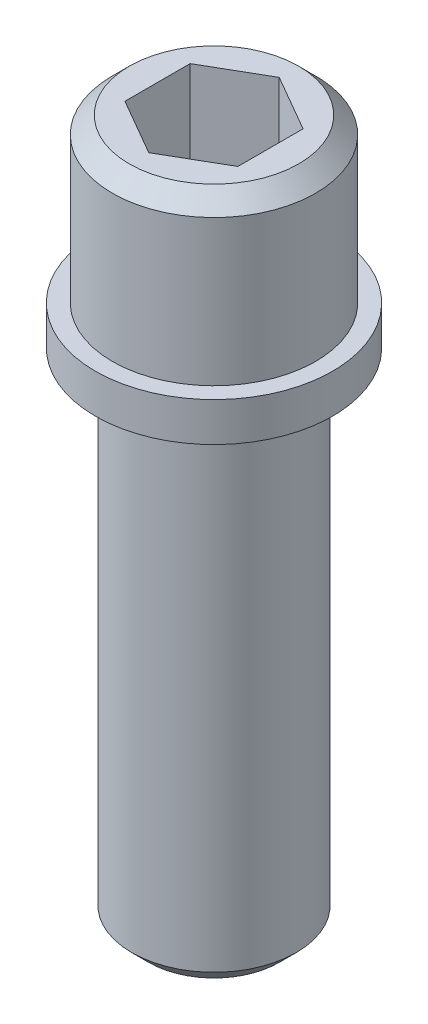
ISO-10303-21;
HEADER;
FILE_DESCRIPTION(('STEP AP214'),'2;1');
FILE_NAME('part.step','',(''),(''),'','','');
FILE_SCHEMA(('AUTOMOTIVE_DESIGN { 1 0 10303 214 1 1 1 1 }'));
ENDSEC;
DATA;
#1=APPLICATION_CONTEXT('core data for automotive mechanical design processes');
#2=APPLICATION_PROTOCOL_DEFINITION('international standard','automotive_design',2000,#1);
#3=PRODUCT_CONTEXT('',#1,'mechanical');
#4=PRODUCT('Part','Part','',(#3));
#5=PRODUCT_RELATED_PRODUCT_CATEGORY('part','',(#4));
#6=PRODUCT_DEFINITION_FORMATION('','',#4);
#7=PRODUCT_DEFINITION_CONTEXT('part definition',#1,'design');
#8=PRODUCT_DEFINITION('design','',#6,#7);
#9=PRODUCT_DEFINITION_SHAPE('','',#8);
#10=(LENGTH_UNIT() NAMED_UNIT(*) SI_UNIT(.MILLI.,.METRE.));
#11=(NAMED_UNIT(*) PLANE_ANGLE_UNIT() SI_UNIT($,.RADIAN.));
#12=(NAMED_UNIT(*) SI_UNIT($,.STERADIAN.) SOLID_ANGLE_UNIT());
#13=UNCERTAINTY_MEASURE_WITH_UNIT(LENGTH_MEASURE(1.E-05),#10,'distance_accuracy_value','');
#14=(GEOMETRIC_REPRESENTATION_CONTEXT(3) GLOBAL_UNCERTAINTY_ASSIGNED_CONTEXT((#13)) GLOBAL_UNIT_ASSIGNED_CONTEXT((#10,
#11,#12)) REPRESENTATION_CONTEXT('',''));
#15=CARTESIAN_POINT('',(0.,0.,0.));
#16=DIRECTION('',(0.,0.,1.));
#17=DIRECTION('',(1.,0.,0.));
#18=AXIS2_PLACEMENT_3D('',#15,#16,#17);
#19=CARTESIAN_POINT('',(0.,29.5,0.));
#20=DIRECTION('',(0.,-1.,0.));
#21=DIRECTION('',(0.,0.,-1.));
#22=AXIS2_PLACEMENT_3D('',#19,#20,#21);
#23=CYLINDRICAL_SURFACE('',#22,4.85);
#24=CARTESIAN_POINT('',(0.,1.,0.));
#25=DIRECTION('',(0.,1.,0.));
#26=DIRECTION('',(0.,0.,1.));
#27=AXIS2_PLACEMENT_3D('',#24,#25,#26);
#28=CIRCLE('',#27,4.85);
#29=CARTESIAN_POINT('',(0.,1.,4.85));
#30=VERTEX_POINT('',#29);
#31=EDGE_CURVE('E49',#30,#30,#28,.T.);
#32=ORIENTED_EDGE('',*,*,#31,.T.);
#33=EDGE_LOOP('',(#32));
#34=FACE_BOUND('',#33,.T.);
#35=CARTESIAN_POINT('',(0.,29.5,0.));
#36=DIRECTION('',(0.,1.,0.));
#37=DIRECTION('',(0.,0.,1.));
#38=AXIS2_PLACEMENT_3D('',#35,#36,#37);
#39=CIRCLE('',#38,4.85);
#40=CARTESIAN_POINT('',(0.,29.5,4.85));
#41=VERTEX_POINT('',#40);
#42=EDGE_CURVE('E152',#41,#41,#39,.T.);
#43=ORIENTED_EDGE('',*,*,#42,.F.);
#44=EDGE_LOOP('',(#43));
#45=FACE_BOUND('',#44,.T.);
#46=ADVANCED_FACE('F41',(#34,#45),#23,.T.);
#47=CARTESIAN_POINT('',(0.,0.,0.));
#48=DIRECTION('',(0.,1.,0.));
#49=DIRECTION('',(0.,0.,1.));
#50=AXIS2_PLACEMENT_3D('',#47,#48,#49);
#51=PLANE('',#50);
#52=CARTESIAN_POINT('',(0.,0.,0.));
#53=DIRECTION('',(0.,1.,0.));
#54=DIRECTION('',(0.,0.,1.));
#55=AXIS2_PLACEMENT_3D('',#52,#53,#54);
#56=CIRCLE('',#55,3.84999999999999);
#57=CARTESIAN_POINT('',(0.,0.,3.84999999999999));
#58=VERTEX_POINT('',#57);
#59=EDGE_CURVE('E11',#58,#58,#56,.F.);
#60=ORIENTED_EDGE('',*,*,#59,.T.);
#61=EDGE_LOOP('',(#60));
#62=FACE_BOUND('',#61,.T.);
#63=ADVANCED_FACE('F181',(#62),#51,.F.);
#64=CARTESIAN_POINT('',(0.,31.8,0.));
#65=DIRECTION('',(0.,-1.,0.));
#66=DIRECTION('',(0.,0.,-1.));
#67=AXIS2_PLACEMENT_3D('',#64,#65,#66);
#68=CYLINDRICAL_SURFACE('',#67,7.);
#69=CARTESIAN_POINT('',(0.,31.8,0.));
#70=DIRECTION('',(0.,1.,0.));
#71=DIRECTION('',(0.,0.,1.));
#72=AXIS2_PLACEMENT_3D('',#69,#70,#71);
#73=CIRCLE('',#72,7.);
#74=CARTESIAN_POINT('',(0.,31.8,7.));
#75=VERTEX_POINT('',#74);
#76=EDGE_CURVE('E154',#75,#75,#73,.T.);
#77=ORIENTED_EDGE('',*,*,#76,.F.);
#78=EDGE_LOOP('',(#77));
#79=FACE_BOUND('',#78,.T.);
#80=CARTESIAN_POINT('',(0.,29.5,0.));
#81=DIRECTION('',(0.,1.,0.));
#82=DIRECTION('',(0.,0.,1.));
#83=AXIS2_PLACEMENT_3D('',#80,#81,#82);
#84=CIRCLE('',#83,7.);
#85=CARTESIAN_POINT('',(0.,29.5,7.));
#86=VERTEX_POINT('',#85);
#87=EDGE_CURVE('E144',#86,#86,#84,.T.);
#88=ORIENTED_EDGE('',*,*,#87,.T.);
#89=EDGE_LOOP('',(#88));
#90=FACE_BOUND('',#89,.T.);
#91=ADVANCED_FACE('F184',(#79,#90),#68,.T.);
#92=CARTESIAN_POINT('',(0.,31.8,0.));
#93=DIRECTION('',(0.,1.,0.));
#94=DIRECTION('',(0.,0.,1.));
#95=AXIS2_PLACEMENT_3D('',#92,#93,#94);
#96=PLANE('',#95);
#97=CARTESIAN_POINT('',(0.,31.8,0.));
#98=DIRECTION('',(0.,1.,0.));
#99=DIRECTION('',(0.,0.,1.));
#100=AXIS2_PLACEMENT_3D('',#97,#98,#99);
#101=CIRCLE('',#100,6.);
#102=CARTESIAN_POINT('',(0.,31.8,6.));
#103=VERTEX_POINT('',#102);
#104=EDGE_CURVE('E148',#103,#103,#101,.T.);
#105=ORIENTED_EDGE('',*,*,#104,.F.);
#106=EDGE_LOOP('',(#105));
#107=FACE_BOUND('',#106,.T.);
#108=ORIENTED_EDGE('',*,*,#76,.T.);
#109=EDGE_LOOP('',(#108));
#110=FACE_BOUND('',#109,.T.);
#111=ADVANCED_FACE('F196',(#107,#110),#96,.T.);
#112=CARTESIAN_POINT('',(0.,29.5,0.));
#113=DIRECTION('',(0.,1.,0.));
#114=DIRECTION('',(0.,0.,1.));
#115=AXIS2_PLACEMENT_3D('',#112,#113,#114);
#116=PLANE('',#115);
#117=ORIENTED_EDGE('',*,*,#42,.T.);
#118=EDGE_LOOP('',(#117));
#119=FACE_BOUND('',#118,.T.);
#120=ORIENTED_EDGE('',*,*,#87,.F.);
#121=EDGE_LOOP('',(#120));
#122=FACE_BOUND('',#121,.T.);
#123=ADVANCED_FACE('F198',(#119,#122),#116,.F.);
#124=CARTESIAN_POINT('',(0.,41.4,0.));
#125=DIRECTION('',(0.,-1.,0.));
#126=DIRECTION('',(0.,0.,-1.));
#127=AXIS2_PLACEMENT_3D('',#124,#125,#126);
#128=CYLINDRICAL_SURFACE('',#127,6.);
#129=CARTESIAN_POINT('',(0.,40.4,0.));
#130=DIRECTION('',(0.,1.,0.));
#131=DIRECTION('',(0.,0.,1.));
#132=AXIS2_PLACEMENT_3D('',#129,#130,#131);
#133=CIRCLE('',#132,6.);
#134=CARTESIAN_POINT('',(0.,40.4,6.));
#135=VERTEX_POINT('',#134);
#136=EDGE_CURVE('E165',#135,#135,#133,.F.);
#137=ORIENTED_EDGE('',*,*,#136,.T.);
#138=EDGE_LOOP('',(#137));
#139=FACE_BOUND('',#138,.T.);
#140=ORIENTED_EDGE('',*,*,#104,.T.);
#141=EDGE_LOOP('',(#140));
#142=FACE_BOUND('',#141,.T.);
#143=ADVANCED_FACE('F201',(#139,#142),#128,.T.);
#144=CARTESIAN_POINT('',(0.,41.4,0.));
#145=DIRECTION('',(0.,1.,0.));
#146=DIRECTION('',(0.,0.,1.));
#147=AXIS2_PLACEMENT_3D('',#144,#145,#146);
#148=PLANE('',#147);
#149=CARTESIAN_POINT('',(0.,41.4,0.));
#150=DIRECTION('',(0.,1.,0.));
#151=DIRECTION('',(0.,0.,1.));
#152=AXIS2_PLACEMENT_3D('',#149,#150,#151);
#153=CIRCLE('',#152,5.);
#154=CARTESIAN_POINT('',(0.,41.4,5.));
#155=VERTEX_POINT('',#154);
#156=EDGE_CURVE('E153',#155,#155,#153,.T.);
#157=ORIENTED_EDGE('',*,*,#156,.T.);
#158=EDGE_LOOP('',(#157));
#159=FACE_BOUND('',#158,.T.);
#160=DIRECTION('',(-0.866025403784439,0.,-0.5));
#161=VECTOR('',#160,1.);
#162=CARTESIAN_POINT('',(3.33419780457009,41.4,-1.925));
#163=LINE('',#162,#161);
#164=CARTESIAN_POINT('',(3.33419780457009,41.4,-1.925));
#165=VERTEX_POINT('',#164);
#166=CARTESIAN_POINT('',(0.,41.4,-3.85));
#167=VERTEX_POINT('',#166);
#168=EDGE_CURVE('E60',#165,#167,#163,.T.);
#169=ORIENTED_EDGE('',*,*,#168,.F.);
#170=DIRECTION('',(0.,0.,-1.));
#171=VECTOR('',#170,1.);
#172=CARTESIAN_POINT('',(3.33419780457009,41.4,1.925));
#173=LINE('',#172,#171);
#174=CARTESIAN_POINT('',(3.33419780457009,41.4,1.925));
#175=VERTEX_POINT('',#174);
#176=EDGE_CURVE('E140',#175,#165,#173,.T.);
#177=ORIENTED_EDGE('',*,*,#176,.F.);
#178=DIRECTION('',(0.866025403784439,0.,-0.5));
#179=VECTOR('',#178,1.);
#180=CARTESIAN_POINT('',(0.,41.4,3.85));
#181=LINE('',#180,#179);
#182=CARTESIAN_POINT('',(0.,41.4,3.85));
#183=VERTEX_POINT('',#182);
#184=EDGE_CURVE('E139',#183,#175,#181,.T.);
#185=ORIENTED_EDGE('',*,*,#184,.F.);
#186=DIRECTION('',(0.866025403784439,0.,0.5));
#187=VECTOR('',#186,1.);
#188=CARTESIAN_POINT('',(-3.33419780457009,41.4,1.925));
#189=LINE('',#188,#187);
#190=CARTESIAN_POINT('',(-3.33419780457009,41.4,1.925));
#191=VERTEX_POINT('',#190);
#192=EDGE_CURVE('E102',#191,#183,#189,.T.);
#193=ORIENTED_EDGE('',*,*,#192,.F.);
#194=DIRECTION('',(0.,0.,1.));
#195=VECTOR('',#194,1.);
#196=CARTESIAN_POINT('',(-3.33419780457009,41.4,-1.925));
#197=LINE('',#196,#195);
#198=CARTESIAN_POINT('',(-3.33419780457009,41.4,-1.925));
#199=VERTEX_POINT('',#198);
#200=EDGE_CURVE('E132',#199,#191,#197,.T.);
#201=ORIENTED_EDGE('',*,*,#200,.F.);
#202=DIRECTION('',(-0.866025403784438,0.,0.5));
#203=VECTOR('',#202,1.);
#204=CARTESIAN_POINT('',(0.,41.4,-3.85));
#205=LINE('',#204,#203);
#206=EDGE_CURVE('E131',#167,#199,#205,.T.);
#207=ORIENTED_EDGE('',*,*,#206,.F.);
#208=EDGE_LOOP('',(#169,#177,#185,#193,#201,#207));
#209=FACE_BOUND('',#208,.T.);
#210=ADVANCED_FACE('F206',(#159,#209),#148,.T.);
#211=CARTESIAN_POINT('',(3.33419780457009,31.8,-1.925));
#212=DIRECTION('',(0.5,0.,-0.866025403784439));
#213=DIRECTION('',(-0.866025403784439,0.,-0.5));
#214=AXIS2_PLACEMENT_3D('',#211,#212,#213);
#215=PLANE('',#214);
#216=ORIENTED_EDGE('',*,*,#168,.T.);
#217=DIRECTION('',(0.,1.,0.));
#218=VECTOR('',#217,1.);
#219=CARTESIAN_POINT('',(0.,31.8,-3.85));
#220=LINE('',#219,#218);
#221=CARTESIAN_POINT('',(0.,31.8,-3.85));
#222=VERTEX_POINT('',#221);
#223=EDGE_CURVE('E90',#222,#167,#220,.T.);
#224=ORIENTED_EDGE('',*,*,#223,.F.);
#225=DIRECTION('',(-0.866025403784439,0.,-0.5));
#226=VECTOR('',#225,1.);
#227=CARTESIAN_POINT('',(3.33419780457009,31.8,-1.925));
#228=LINE('',#227,#226);
#229=CARTESIAN_POINT('',(3.33419780457009,31.8,-1.925));
#230=VERTEX_POINT('',#229);
#231=EDGE_CURVE('E145',#230,#222,#228,.T.);
#232=ORIENTED_EDGE('',*,*,#231,.F.);
#233=DIRECTION('',(0.,1.,0.));
#234=VECTOR('',#233,1.);
#235=CARTESIAN_POINT('',(3.33419780457009,31.8,-1.925));
#236=LINE('',#235,#234);
#237=EDGE_CURVE('E63',#230,#165,#236,.T.);
#238=ORIENTED_EDGE('',*,*,#237,.T.);
#239=EDGE_LOOP('',(#216,#224,#232,#238));
#240=FACE_BOUND('',#239,.T.);
#241=ADVANCED_FACE('F215',(#240),#215,.F.);
#242=CARTESIAN_POINT('',(3.33419780457009,31.8,1.925));
#243=DIRECTION('',(1.,0.,0.));
#244=DIRECTION('',(0.,0.,-1.));
#245=AXIS2_PLACEMENT_3D('',#242,#243,#244);
#246=PLANE('',#245);
#247=ORIENTED_EDGE('',*,*,#176,.T.);
#248=ORIENTED_EDGE('',*,*,#237,.F.);
#249=DIRECTION('',(0.,0.,-1.));
#250=VECTOR('',#249,1.);
#251=CARTESIAN_POINT('',(3.33419780457009,31.8,1.925));
#252=LINE('',#251,#250);
#253=CARTESIAN_POINT('',(3.33419780457009,31.8,1.925));
#254=VERTEX_POINT('',#253);
#255=EDGE_CURVE('E120',#254,#230,#252,.T.);
#256=ORIENTED_EDGE('',*,*,#255,.F.);
#257=DIRECTION('',(0.,1.,0.));
#258=VECTOR('',#257,1.);
#259=CARTESIAN_POINT('',(3.33419780457009,31.8,1.925));
#260=LINE('',#259,#258);
#261=EDGE_CURVE('E107',#254,#175,#260,.T.);
#262=ORIENTED_EDGE('',*,*,#261,.T.);
#263=EDGE_LOOP('',(#247,#248,#256,#262));
#264=FACE_BOUND('',#263,.T.);
#265=ADVANCED_FACE('F216',(#264),#246,.F.);
#266=CARTESIAN_POINT('',(0.,31.8,3.85));
#267=DIRECTION('',(0.5,0.,0.866025403784439));
#268=DIRECTION('',(0.866025403784439,0.,-0.5));
#269=AXIS2_PLACEMENT_3D('',#266,#267,#268);
#270=PLANE('',#269);
#271=ORIENTED_EDGE('',*,*,#184,.T.);
#272=ORIENTED_EDGE('',*,*,#261,.F.);
#273=DIRECTION('',(0.866025403784439,0.,-0.5));
#274=VECTOR('',#273,1.);
#275=CARTESIAN_POINT('',(0.,31.8,3.85));
#276=LINE('',#275,#274);
#277=CARTESIAN_POINT('',(0.,31.8,3.85));
#278=VERTEX_POINT('',#277);
#279=EDGE_CURVE('E113',#278,#254,#276,.T.);
#280=ORIENTED_EDGE('',*,*,#279,.F.);
#281=DIRECTION('',(0.,1.,0.));
#282=VECTOR('',#281,1.);
#283=CARTESIAN_POINT('',(0.,31.8,3.85));
#284=LINE('',#283,#282);
#285=EDGE_CURVE('E96',#278,#183,#284,.T.);
#286=ORIENTED_EDGE('',*,*,#285,.T.);
#287=EDGE_LOOP('',(#271,#272,#280,#286));
#288=FACE_BOUND('',#287,.T.);
#289=ADVANCED_FACE('F112',(#288),#270,.F.);
#290=CARTESIAN_POINT('',(-3.33419780457009,31.8,1.925));
#291=DIRECTION('',(-0.5,0.,0.866025403784439));
#292=DIRECTION('',(0.866025403784439,0.,0.5));
#293=AXIS2_PLACEMENT_3D('',#290,#291,#292);
#294=PLANE('',#293);
#295=ORIENTED_EDGE('',*,*,#192,.T.);
#296=ORIENTED_EDGE('',*,*,#285,.F.);
#297=DIRECTION('',(0.866025403784439,0.,0.5));
#298=VECTOR('',#297,1.);
#299=CARTESIAN_POINT('',(-3.33419780457009,31.8,1.925));
#300=LINE('',#299,#298);
#301=CARTESIAN_POINT('',(-3.33419780457009,31.8,1.925));
#302=VERTEX_POINT('',#301);
#303=EDGE_CURVE('E105',#302,#278,#300,.T.);
#304=ORIENTED_EDGE('',*,*,#303,.F.);
#305=DIRECTION('',(0.,1.,0.));
#306=VECTOR('',#305,1.);
#307=CARTESIAN_POINT('',(-3.33419780457009,31.8,1.925));
#308=LINE('',#307,#306);
#309=EDGE_CURVE('E109',#302,#191,#308,.T.);
#310=ORIENTED_EDGE('',*,*,#309,.T.);
#311=EDGE_LOOP('',(#295,#296,#304,#310));
#312=FACE_BOUND('',#311,.T.);
#313=ADVANCED_FACE('F99',(#312),#294,.F.);
#314=CARTESIAN_POINT('',(-3.33419780457009,31.8,-1.925));
#315=DIRECTION('',(-1.,0.,0.));
#316=DIRECTION('',(0.,0.,1.));
#317=AXIS2_PLACEMENT_3D('',#314,#315,#316);
#318=PLANE('',#317);
#319=ORIENTED_EDGE('',*,*,#200,.T.);
#320=ORIENTED_EDGE('',*,*,#309,.F.);
#321=DIRECTION('',(0.,0.,1.));
#322=VECTOR('',#321,1.);
#323=CARTESIAN_POINT('',(-3.33419780457009,31.8,-1.925));
#324=LINE('',#323,#322);
#325=CARTESIAN_POINT('',(-3.33419780457009,31.8,-1.925));
#326=VERTEX_POINT('',#325);
#327=EDGE_CURVE('E124',#326,#302,#324,.T.);
#328=ORIENTED_EDGE('',*,*,#327,.F.);
#329=DIRECTION('',(0.,1.,0.));
#330=VECTOR('',#329,1.);
#331=CARTESIAN_POINT('',(-3.33419780457009,31.8,-1.925));
#332=LINE('',#331,#330);
#333=EDGE_CURVE('E150',#326,#199,#332,.T.);
#334=ORIENTED_EDGE('',*,*,#333,.T.);
#335=EDGE_LOOP('',(#319,#320,#328,#334));
#336=FACE_BOUND('',#335,.T.);
#337=ADVANCED_FACE('F219',(#336),#318,.F.);
#338=CARTESIAN_POINT('',(0.,31.8,-3.85));
#339=DIRECTION('',(-0.5,0.,-0.866025403784439));
#340=DIRECTION('',(-0.866025403784439,0.,0.5));
#341=AXIS2_PLACEMENT_3D('',#338,#339,#340);
#342=PLANE('',#341);
#343=ORIENTED_EDGE('',*,*,#206,.T.);
#344=ORIENTED_EDGE('',*,*,#333,.F.);
#345=DIRECTION('',(-0.866025403784438,0.,0.5));
#346=VECTOR('',#345,1.);
#347=CARTESIAN_POINT('',(0.,31.8,-3.85));
#348=LINE('',#347,#346);
#349=EDGE_CURVE('E123',#222,#326,#348,.T.);
#350=ORIENTED_EDGE('',*,*,#349,.F.);
#351=ORIENTED_EDGE('',*,*,#223,.T.);
#352=EDGE_LOOP('',(#343,#344,#350,#351));
#353=FACE_BOUND('',#352,.T.);
#354=ADVANCED_FACE('F220',(#353),#342,.F.);
#355=CARTESIAN_POINT('',(0.,31.8,0.));
#356=DIRECTION('',(0.,1.,0.));
#357=DIRECTION('',(0.,0.,1.));
#358=AXIS2_PLACEMENT_3D('',#355,#356,#357);
#359=PLANE('',#358);
#360=ORIENTED_EDGE('',*,*,#231,.T.);
#361=ORIENTED_EDGE('',*,*,#349,.T.);
#362=ORIENTED_EDGE('',*,*,#327,.T.);
#363=ORIENTED_EDGE('',*,*,#303,.T.);
#364=ORIENTED_EDGE('',*,*,#279,.T.);
#365=ORIENTED_EDGE('',*,*,#255,.T.);
#366=EDGE_LOOP('',(#360,#361,#362,#363,#364,#365));
#367=FACE_BOUND('',#366,.T.);
#368=ADVANCED_FACE('F119',(#367),#359,.T.);
#369=CARTESIAN_POINT('',(0.,41.4,0.));
#370=DIRECTION('',(0.,-1.,0.));
#371=DIRECTION('',(0.,0.,-1.));
#372=AXIS2_PLACEMENT_3D('',#369,#370,#371);
#373=CONICAL_SURFACE('',#372,5.,0.785398163397446);
#374=ORIENTED_EDGE('',*,*,#136,.F.);
#375=EDGE_LOOP('',(#374));
#376=FACE_BOUND('',#375,.T.);
#377=ORIENTED_EDGE('',*,*,#156,.F.);
#378=EDGE_LOOP('',(#377));
#379=FACE_BOUND('',#378,.T.);
#380=ADVANCED_FACE('F175',(#376,#379),#373,.T.);
#381=CARTESIAN_POINT('',(0.,1.,0.));
#382=DIRECTION('',(0.,1.,0.));
#383=DIRECTION('',(0.,0.,1.));
#384=AXIS2_PLACEMENT_3D('',#381,#382,#383);
#385=CONICAL_SURFACE('',#384,4.85,0.785398163397452);
#386=ORIENTED_EDGE('',*,*,#59,.F.);
#387=EDGE_LOOP('',(#386));
#388=FACE_BOUND('',#387,.T.);
#389=ORIENTED_EDGE('',*,*,#31,.F.);
#390=EDGE_LOOP('',(#389));
#391=FACE_BOUND('',#390,.T.);
#392=ADVANCED_FACE('F42',(#388,#391),#385,.T.);
#393=CLOSED_SHELL('',(#46,#63,#91,#111,#123,#143,#210,#241,#265,#289,#313,#337,#354,#368,#380,#392));
#394=MANIFOLD_SOLID_BREP('B2',#393);
#395=ADVANCED_BREP_SHAPE_REPRESENTATION('',(#18,#394),#14);
#396=SHAPE_DEFINITION_REPRESENTATION(#9,#395);
ENDSEC;
END-ISO-10303-21;
